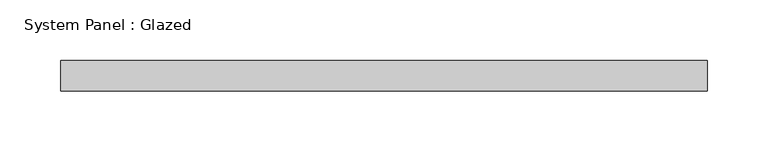
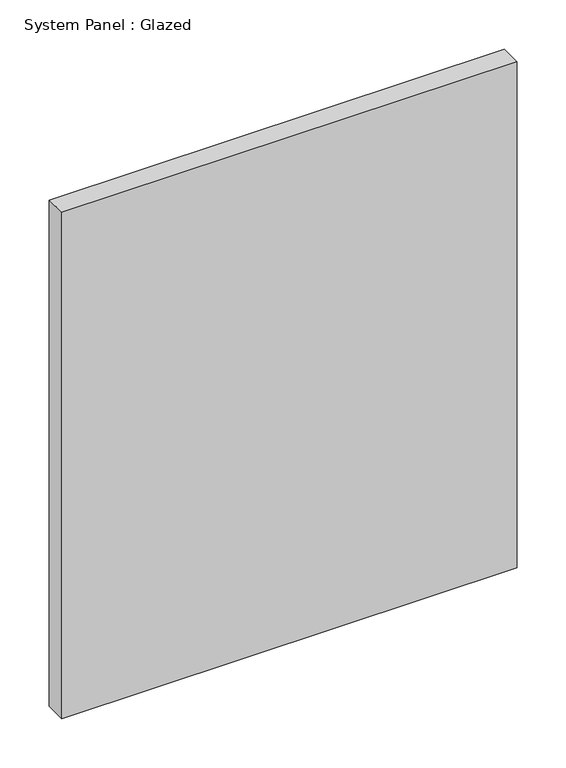
"""IFC4 building model written with IfcOpenShell, lengths in millimetres: plate geometry, System Panel : Glazed."""

from ifc_helpers import new_model, si_unit, origin, origin_with_axes, place, context, project, spatial, polyline, outline, extrude, source, transform, mapped, element, save


def system_panel_glazed_68ae91f2(model_context):
    return source(origin(), model_context, "Body", "SweptSolid", [
        extrude(outline(polyline([(266.7, 19.05), (-266.7, 19.05), (-266.7, 44.45), (266.7, 44.45), (266.7, 19.05)])), origin_with_axes(), (0.0, 0.0, 1.0), 626.9740338),
    ])


if __name__ == "__main__":
    model = new_model("IFC4")
    model_context = context("Model", 3, world=origin())
    ifc_project = project(units=[si_unit("LENGTHUNIT", "METRE", prefix="MILLI")], contexts=[model_context])
    site = spatial("IfcSite", under=ifc_project)
    building = spatial("IfcBuilding", under=site)
    placement = place(None, origin())
    system_panel_glazed_shape = system_panel_glazed_68ae91f2(model_context)
    element("IfcPlate", 1, ObjectType="System Panel : Glazed", at=placement, inside=building, context=model_context, shape_type="MappedRepresentation", body=[
        mapped(system_panel_glazed_shape, transform((0.0, 0.0, 0.0), x_axis=(1.0, 0.0, 0.0), y_axis=(0.0, 1.0, 0.0), z_axis=(0.0, 0.0, 1.0))),
    ])
    save(model, "model.ifc")

# Revit data of these elements
# Type "System Panel : Glazed"
#   Construction Type Id = "GSP4R"
#   Analytic Construction = "1/8 in Pilkington single glazing"
#   Visual Light Transmittance = 0.9
#   Solar Heat Gain Coefficient = 0.86
#   Heat Transfer Coefficient (U) = 1.18115 BTU/(h·ft²·°F)
#   Define Thermal Properties by = 1
# Element 1 (IfcPlate, "System Panel : Glazed")
#   Materials on its faces: "Glass"
# Materials
#   "Glass": class "Glass", colour RGB 0 128 192, transparency 0.75, Description = "Soda Lime Glass", Cost = 0
